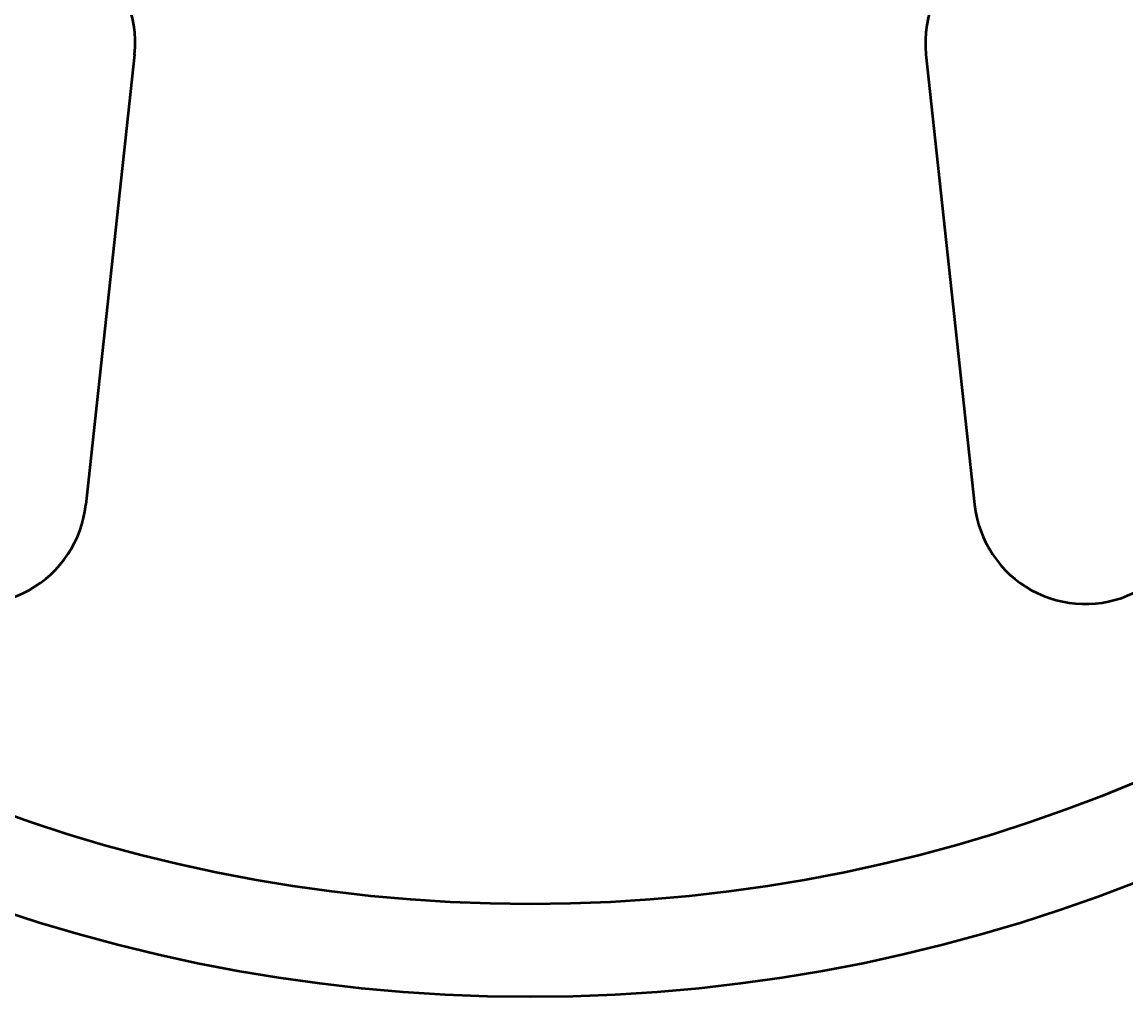
# Model space of a CAD drawing. Units: inches. Extents: x -99 to 284, y -92 to 134.
# Tile 2 of 16: x 5 to 64, y -74 to -22. Entities that reach past the tile are written whole.
import ezdxf

# ---------------------------------------------------------------- set-up
doc = ezdxf.new("R2010")
doc.units = ezdxf.units.IN
doc.header["$MEASUREMENT"] = 0
doc.layers.add('M-DIMS', color=2, linetype='Continuous', lineweight=18)
doc.layers.add('M-OUTL', color=7, linetype='Continuous', lineweight=50)
doc.styles.get("Standard").update_dxf_attribs({"font": 'arial.ttf'})
doc.dimstyles.get("Standard").update_dxf_attribs({"dimtxt": 0.18, "dimasz": 0.18, "dimexe": 0.18, "dimexo": 0.0625, "dimgap": 0.09, "dimtad": 0, "dimtih": 1, "dimtoh": 1, "dimdec": 4, "dimzin": 0, "dimdsep": 46, "dimtxsty": 'Standard', "dimcen": 0.09, "dimadec": 0, "dimazin": 0, "dimtfac": 1, "dimtdec": 4, "dimtofl": 0, "dimtmove": 0, "dimatfit": 3, "dimfxl": 1, "dimtolj": 1, "dimtzin": 0, "dimarcsym": 0})

# ---------------------------------------------------------------- blocks, each defined once
blk = doc.blocks.new('*U1')
for p, q in [((-5.205, -13.52), (-17.34, 7.646)), ((5.205, -13.52), (17.34, 7.646))]:
    blk.add_line(p, q)
for centre, start, end in [((-12.135, 10.63), 100.17697, 209.82635), ((12.135, 10.63), 330.17365, 79.82303), ((0, -10.536), 209.82635, 330.17365)]:
    blk.add_arc(centre, 6, start, end)
blk = doc.blocks.new('*U2')
at = {"layer": 'M-OUTL', "color": 0, "linetype": 'ByBlock', "lineweight": -2, "transparency": 16777216}
for p, rotation in [((-1.509, -31.235), 144), ((65.462, -31.235), 216)]:
    blk.add_blockref('*U1', p, dxfattribs=dict(at, rotation=rotation))
blk = doc.blocks.new('*D19')
at = {"layer": 'Defpoints', "color": 0, "transparency": 16777216}
for p in [(112.982, 51.721), (-49.029, -22.013)]:
    blk.add_point(p, dxfattribs=at)
at = {"layer": 'M-DIMS', "color": 0, "lineweight": -2, "transparency": 16777216}
for p, q in [((31.976, 14.764), (31.976, 14.944)), ((31.886, 14.854), (32.066, 14.854)), ((-97.632, -44.133), (-49.192, -22.088)), ((-97.812, -44.133), (-97.632, -44.133))]:
    blk.add_line(p, q, dxfattribs=at)
at = {"layer": 'M-DIMS', "color": 0, "transparency": 16777216}
blk.add_solid([(-49.205, -22.06), (-49.18, -22.115), (-49.029, -22.013)], dxfattribs=at)
at = {"layer": 'M-DIMS', "color": 0, "transparency": 16777216, "insert": (-98.199, -44.133), "char_height": 0.18, "attachment_point": 5}
blk.add_mtext('\\A1;∅178', dxfattribs=at)
blk = doc.blocks.new('*D20')
at = {"layer": 'Defpoints', "color": 0, "transparency": 16777216}
for p in [(-35.23, 65.245), (99.183, -35.537)]:
    blk.add_point(p, dxfattribs=at)
at = {"layer": 'M-DIMS', "color": 0, "lineweight": -2, "transparency": 16777216}
for p, q in [((31.976, 14.764), (31.976, 14.944)), ((31.886, 14.854), (32.066, 14.854)), ((139.507, -65.772), (99.327, -35.645)), ((139.687, -65.772), (139.507, -65.772))]:
    blk.add_line(p, q, dxfattribs=at)
at = {"layer": 'M-DIMS', "color": 0, "transparency": 16777216}
blk.add_solid([(99.345, -35.621), (99.309, -35.669), (99.183, -35.537)], dxfattribs=at)
at = {"layer": 'M-DIMS', "color": 0, "transparency": 16777216, "insert": (140.074, -65.772), "char_height": 0.18, "attachment_point": 5}
blk.add_mtext('\\A1;∅168', dxfattribs=at)

msp = doc.modelspace()

# ---------------------------------------------------------------- linework, layer by layer
at = {"layer": 'M-OUTL'}
for radius in [89, 84]:
    msp.add_circle((31.9765, 14.8539), radius, dxfattribs=at)

# ---------------------------------------------------------------- block references
msp.add_blockref('*U2', (0, 0), dxfattribs=at)

# ---------------------------------------------------------------- dimensions: what is measured, and where the dimension line sits
at = {"layer": 'M-DIMS'}
for p1, p2, picture, middle in [((-35.2301, 65.2451), (99.1831, -35.5373), '*D20', (140.074, -65.772)), ((112.9816, 51.7208), (-49.0286, -22.013), '*D19', (-98.1987, -44.1332))]:
    dim = msp.add_diameter_dim_2p(p1=p1, p2=p2, dimstyle='Standard', override={"dimdec": 0, "dimlfac": 1, "dimrnd": 0, "dimzin": 0, "dimdsep": 46, "dimlunit": 2}, dxfattribs=at)
    dim.commit()
    dim.dimension.update_dxf_attribs({"geometry": picture, "text_midpoint": middle, "dimtype": 163})

doc.saveas('drawing.dxf')
